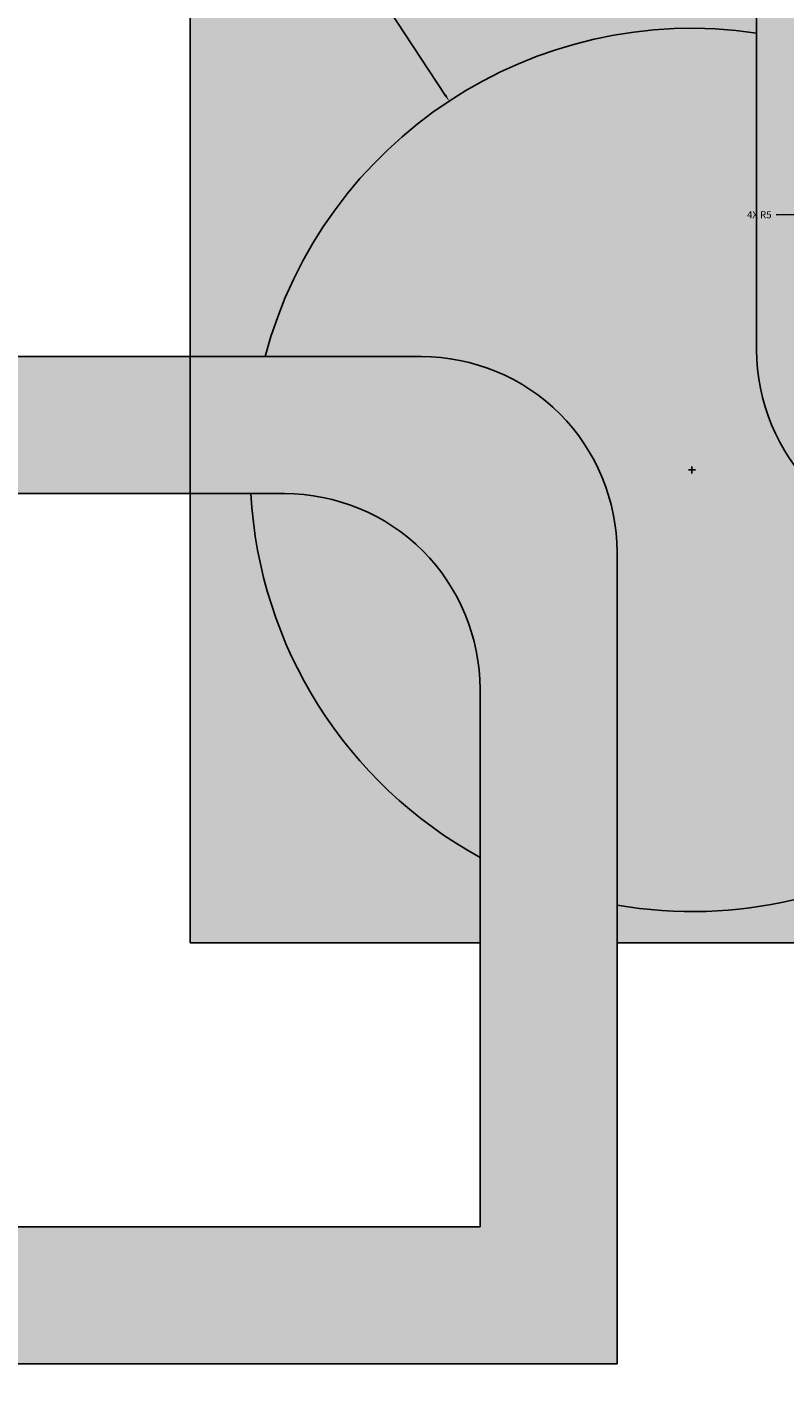
# Model space of a CAD drawing. Units: millimetres. Extents: x -11 to 280, y -4 to 208.
# Tile 30 of 55: x 170 to 189, y 54 to 88. Entities that reach past the tile are written whole.
import ezdxf

# ---------------------------------------------------------------- set-up
doc = ezdxf.new("R2010")
doc.units = ezdxf.units.MM
for name, color, linetype, lineweight in [('M-DIMS', 2, 'Continuous', 18), ('M-HYDR-PRES', 7, 'Continuous', 25), ('M-HYDR-RETN', 7, 'Continuous', 25), ('M-HYDR-VALV', 7, 'Continuous', 25), ('M-HYDR-VALV-PATT', 252, 'Continuous', 13)]:
    doc.layers.add(name, color=color, linetype=linetype, lineweight=lineweight)
doc.layers.add('M-HYDR-PRES-PATT', color=240, linetype='Continuous', lineweight=13, true_color=0xed1f24)
doc.layers.add('M-HYDR-RETN-PATT', color=114, linetype='Continuous', lineweight=13, true_color=0x139b48)
doc.styles.get("Standard").update_dxf_attribs({"font": 'arial.ttf'})
doc.dimstyles.get("Standard").update_dxf_attribs({"dimtxt": 0.18, "dimasz": 0.18, "dimexe": 0.18, "dimexo": 0.0625, "dimgap": 0.09, "dimtad": 0, "dimtih": 1, "dimtoh": 1, "dimdec": 4, "dimzin": 0, "dimdsep": 46, "dimtxsty": 'Standard', "dimcen": 0.09, "dimadec": 0, "dimazin": 0, "dimtfac": 1, "dimtdec": 4, "dimtofl": 0, "dimtmove": 0, "dimatfit": 3, "dimfxl": 1, "dimtolj": 1, "dimtzin": 0, "dimarcsym": 0})

# ---------------------------------------------------------------- blocks, each defined once
blk = doc.blocks.new('*D4')
at = {"layer": 'Defpoints', "color": 0, "transparency": 16777216}
for p in [(4.763, 84.426), (266.035, 51.733), (266.035, -3.415)]:
    blk.add_point(p, dxfattribs=at)
at = {"layer": 'M-DIMS', "color": 0, "lineweight": -2, "transparency": 16777216}
for p, q in [((4.763, 84.364), (4.763, -3.595)), ((266.035, 51.67), (266.035, -3.595)), ((4.943, -3.415), (134.934, -3.415)), ((265.855, -3.415), (135.864, -3.415))]:
    blk.add_line(p, q, dxfattribs=at)
at = {"layer": 'M-DIMS', "color": 0, "transparency": 16777216}
for points in [[(4.943, -3.385), (4.943, -3.445), (4.763, -3.415)], [(265.855, -3.385), (265.855, -3.445), (266.035, -3.415)]]:
    blk.add_solid(points, dxfattribs=at)
at = {"layer": 'M-DIMS', "color": 0, "transparency": 16777216, "insert": (135.399, -3.415), "char_height": 0.18, "attachment_point": 5}
blk.add_mtext('\\A1;261.27', dxfattribs=at)
blk = doc.blocks.new('*D5')
at = {"layer": 'Defpoints', "color": 0, "transparency": 16777216}
for p in [(24.759, 192.645), (-10.087, 11.435), (261.686, 11.435)]:
    blk.add_point(p, dxfattribs=at)
at = {"layer": 'M-DIMS', "color": 0, "lineweight": -2, "transparency": 16777216}
for p, q in [((24.696, 192.645), (-10.267, 192.645)), ((-10.087, 192.465), (-10.087, 102.222)), ((-10.087, 11.615), (-10.087, 101.858)), ((261.624, 11.435), (-10.267, 11.435))]:
    blk.add_line(p, q, dxfattribs=at)
at = {"layer": 'M-DIMS', "color": 0, "transparency": 16777216}
for points in [[(-10.117, 192.465), (-10.057, 192.465), (-10.087, 192.645)], [(-10.117, 11.615), (-10.057, 11.615), (-10.087, 11.435)]]:
    blk.add_solid(points, dxfattribs=at)
at = {"layer": 'M-DIMS', "color": 0, "transparency": 16777216, "insert": (-10.087, 102.04), "char_height": 0.18, "attachment_point": 5}
blk.add_mtext('\\A1;181.2', dxfattribs=at)
blk = doc.blocks.new('*D18')
at = {"layer": 'Defpoints', "color": 0, "transparency": 16777216}
for p in [(173.804, 207.495), (173.804, 65.064), (151.022, 43.599)]:
    blk.add_point(p, dxfattribs=at)
at = {"layer": 'M-DIMS', "color": 0, "lineweight": -2, "transparency": 16777216}
for p, q in [((151.022, 43.662), (151.022, 207.675)), ((151.202, 207.495), (162.017, 207.495)), ((173.624, 207.495), (162.808, 207.495)), ((173.804, 65.126), (173.804, 207.675))]:
    blk.add_line(p, q, dxfattribs=at)
at = {"layer": 'M-DIMS', "color": 0, "transparency": 16777216}
for points in [[(151.202, 207.525), (151.202, 207.465), (151.022, 207.495)], [(173.624, 207.525), (173.624, 207.465), (173.804, 207.495)]]:
    blk.add_solid(points, dxfattribs=at)
at = {"layer": 'M-DIMS', "color": 0, "transparency": 16777216, "insert": (162.413, 207.495), "char_height": 0.18, "attachment_point": 5}
blk.add_mtext('\\A1;22.78', dxfattribs=at)
blk = doc.blocks.new('*D20')
at = {"layer": 'Defpoints', "color": 0, "transparency": 16777216}
for p in [(231.68, 207.495), (151.022, 43.599), (231.68, 43.599)]:
    blk.add_point(p, dxfattribs=at)
at = {"layer": 'M-DIMS', "color": 0, "lineweight": -2, "transparency": 16777216}
for p, q in [((151.022, 43.662), (151.022, 207.675)), ((151.202, 207.495), (190.957, 207.495)), ((231.5, 207.495), (191.745, 207.495)), ((231.68, 43.662), (231.68, 207.675))]:
    blk.add_line(p, q, dxfattribs=at)
at = {"layer": 'M-DIMS', "color": 0, "transparency": 16777216}
for points in [[(151.202, 207.525), (151.202, 207.465), (151.022, 207.495)], [(231.5, 207.525), (231.5, 207.465), (231.68, 207.495)]]:
    blk.add_solid(points, dxfattribs=at)
at = {"layer": 'M-DIMS', "color": 0, "transparency": 16777216, "insert": (191.351, 207.495), "char_height": 0.18, "attachment_point": 5}
blk.add_mtext('\\A1;80.66', dxfattribs=at)
blk = doc.blocks.new('*D29')
at = {"layer": 'Defpoints', "color": 0, "transparency": 16777216}
for p in [(180.42, 86.567), (186.62, 77.144)]:
    blk.add_point(p, dxfattribs=at)
at = {"layer": 'M-DIMS', "color": 0, "lineweight": -2, "transparency": 16777216}
for p, q in [((176.52, 92.221), (176.7, 92.221)), ((176.7, 92.221), (180.321, 86.718)), ((186.53, 77.144), (186.71, 77.144)), ((186.62, 77.054), (186.62, 77.234))]:
    blk.add_line(p, q, dxfattribs=at)
at = {"layer": 'M-DIMS', "color": 0, "transparency": 16777216}
blk.add_solid([(180.346, 86.734), (180.296, 86.701), (180.42, 86.567)], dxfattribs=at)
at = {"layer": 'M-DIMS', "color": 0, "transparency": 16777216, "insert": (175.843, 92.221), "char_height": 0.18, "attachment_point": 5}
blk.add_mtext('\\A1;4X R11.28', dxfattribs=at)
blk = doc.blocks.new('*D31')
at = {"layer": 'Defpoints', "color": 0, "transparency": 16777216}
for p in [(191.775, 83.68), (196.774, 83.71)]:
    blk.add_point(p, dxfattribs=at)
at = {"layer": 'M-DIMS', "color": 0, "lineweight": -2, "transparency": 16777216}
for p, q in [((188.775, 83.662), (191.595, 83.679)), ((196.684, 83.71), (196.864, 83.71)), ((196.774, 83.62), (196.774, 83.8))]:
    blk.add_line(p, q, dxfattribs=at)
at = {"layer": 'M-DIMS', "color": 0, "transparency": 16777216}
blk.add_solid([(191.594, 83.709), (191.595, 83.649), (191.775, 83.68)], dxfattribs=at)
at = {"layer": 'M-DIMS', "color": 0, "transparency": 16777216, "insert": (188.342, 83.662), "char_height": 0.18, "attachment_point": 5}
blk.add_mtext('\\A1;4X R5', dxfattribs=at)

msp = doc.modelspace()

# ---------------------------------------------------------------- hatches: boundary and pattern name
at = {"layer": 'M-HYDR-PRES-PATT'}
h = msp.add_hatch(color=256, dxfattribs=at)
h.set_gradient(color1=(237, 31, 36), color2=(237, 31, 36), tint=1)
h.paths.add_polyline_path([(232.2, 133.1228), (228.7, 133.1228), (228.7, 108.8141), (102.7646, 108.8141), (102.7646, 105.3141), (232.2, 105.3141)])
h.paths.add_polyline_path([(128.8433, 105.3141), (125.3433, 105.3141), (125.3433, 91.7099, 1), (128.8433, 91.7099)])
h.paths.add_polyline_path([(229.1617, 78.7098), (196.7745, 78.7098, -0.4142136), (191.7745, 83.7098), (191.7745, 105.3141), (188.2745, 105.3141), (188.2745, 80.2098, 0.4142136), (193.2745, 75.2098), (225.6617, 75.2098), (225.6617, 43.5991), (229.1617, 43.5991)])
h.paths.add_polyline_path([(102.7646, 110.3704), (95.5776, 110.3704), (95.5776, 103.9022), (102.7646, 103.9022)])
h.paths.add_polyline_path([(100.7059, 107.2502), (99.1711, 106.3641), (99.1711, 106.8641), (97.1711, 106.8641), (97.1711, 107.6363), (99.1711, 107.6363), (99.1711, 108.1363)], flags=16)
h.paths.add_polyline_path([(234.6119, 138.4081), (226.5106, 138.4081), (226.5106, 133.1228), (234.6119, 133.1228)])
h.paths.add_polyline_path([(231.1963, 135.7055), (230.2965, 134.1786), (229.4241, 135.7213), (229.9241, 135.7168), (229.9418, 137.7167), (230.7141, 137.7099), (230.6963, 135.71)], flags=16)
at = {"layer": 'M-HYDR-RETN-PATT'}
h = msp.add_hatch(color=256, dxfattribs=at)
h.set_gradient(color1=(19, 155, 72), color2=(19, 155, 72), tint=1)
h.paths.add_polyline_path([(17.9701, 159.0814), (29.2015, 159.0814), (29.2015, 162.5814), (14.4701, 162.5814), (14.4701, 98.0213), (17.9701, 98.0213)])
h.paths.add_polyline_path([(17.9701, 84.4261), (14.4701, 84.4261), (14.4701, 54.3099), (156.2446, 54.3099), (156.2446, 57.8099), (17.9701, 57.8099)])
h.paths.add_polyline_path([(120.5137, 74.3991), (17.9701, 74.3991), (17.9701, 70.8991), (120.5137, 70.8991)], flags=17)
h.paths.add_polyline_path([(184.7092, 75.04, 0.4142136), (179.7092, 80.04), (156.2446, 80.04), (156.2446, 57.8099), (156.2446, 54.3099), (156.2446, 43.5991), (159.7446, 43.5991), (159.7446, 57.8099), (159.7446, 76.54), (176.2092, 76.54, -0.4142136), (181.2092, 71.54), (181.2092, 57.8099), (159.7446, 57.8099), (159.7446, 54.3099), (184.7092, 54.3099)])
at = {"layer": 'M-HYDR-VALV-PATT'}
h = msp.add_hatch(color=256, dxfattribs=at)
h.set_gradient(color1=(153, 27, 30), color2=(153, 27, 30), tint=1)
h.paths.add_polyline_path([(131.8437, 88.2421, -0.3394543), (132.5849, 89.208), (121.2548, 86.1721, -0.4931454), (122.5137, 85.2062, -0.3394543), (121.7725, 84.2403), (133.1025, 87.2762, -0.4931454)])
h.paths.add_polyline_path([(133.1025, 83.1351, -0.4931454), (131.8437, 84.101, -0.3394543), (132.5849, 85.0669), (121.2548, 82.031, -0.4931454), (122.5137, 81.0651, -0.3394543), (121.7725, 80.0992)])
h.paths.add_polyline_path([(133.1025, 78.994, -0.4931454), (131.8437, 79.9599, -0.3394543), (132.5849, 80.9258), (121.2548, 77.8899, -0.4931454), (122.5137, 76.924, -0.3394543), (121.7725, 75.9581)])
h.paths.add_polyline_path([(197.7905, 78.7098), (200.0003, 78.7098), (200.0003, 89.3873), (191.7745, 89.3873), (191.7745, 87.1776, -0.2439164)])
h.paths.add_polyline_path([(200.0003, 65.0638), (200.0003, 75.2098), (197.7325, 75.2098, -0.4135811), (184.7092, 66.0277), (184.7092, 65.0638)])
h.paths.add_polyline_path([(181.2092, 65.0638), (181.2092, 67.2471, -0.2598454), (175.3563, 76.54), (173.8038, 76.54), (173.8038, 65.0638)])
h.paths.add_polyline_path([(188.2745, 88.3022), (188.2745, 89.3873), (173.8038, 89.3873), (173.8038, 80.04), (175.7181, 80.04, -0.3816661)])
h = msp.add_hatch(color=256, dxfattribs=at)
h.set_gradient(color1=(205, 105, 40), color2=(34, 52, 110), tint=1, name='INVCYLINDER')
h.paths.add_polyline_path([(188.2745, 80.2098), (188.2745, 88.3022, 0.3816661), (175.7181, 80.04), (179.7092, 80.04, -0.4142136), (184.7092, 75.04), (184.7092, 66.0277, 0.4135811), (197.7325, 75.2098), (193.2745, 75.2098, -0.4142136)])
h.paths.add_polyline_path([(176.2092, 76.54), (175.3563, 76.54, 0.2598454), (181.2092, 67.2471), (181.2092, 71.54, 0.4142136)])
h.paths.add_polyline_path([(196.7745, 78.7098), (197.7905, 78.7098, 0.2439164), (191.7745, 87.1776), (191.7745, 83.7098, 0.4142136)])

# ---------------------------------------------------------------- linework, layer by layer
at = {"layer": 'M-HYDR-PRES'}
msp.add_lwpolyline([(188.2745, 105.3141), (188.2745, 80.2098, 0.4142136), (193.2745, 75.2098), (225.6617, 75.2098), (225.6617, 43.5991)], format="xyb", dxfattribs=at)
at = {"layer": 'M-HYDR-RETN'}
msp.add_lwpolyline([(159.7446, 54.3099), (184.7092, 54.3099), (184.7092, 75.04, 0.4142136), (179.7092, 80.04), (156.2446, 80.04), (156.2446, 57.8099)], format="xyb", dxfattribs=at)
msp.add_lwpolyline([(159.7446, 57.8099), (181.2092, 57.8099), (181.2092, 71.54, 0.4142136), (176.2092, 76.54), (159.7446, 76.54)], format="xyb", close=True, dxfattribs=at)
at = {"layer": 'M-HYDR-VALV'}
for points in [[(173.8038, 80.04), (173.8038, 89.3873), (188.2745, 89.3873)], [(181.2092, 65.0638), (173.8038, 65.0638), (173.8038, 76.54)], [(200.0003, 75.2098), (200.0003, 65.0638), (184.7092, 65.0638)]]:
    msp.add_lwpolyline(points, dxfattribs=at)
for start, end in [(81.565, 165.12565), (183.07195, 241.33562), (260.24776, 350.12401)]:
    msp.add_arc((186.6199, 77.1445), 11.2798, start, end, dxfattribs=at)

# ---------------------------------------------------------------- dimensions: what is measured, and where the dimension line sits
at = {"layer": 'M-DIMS'}
for base, p1, p2, picture, middle in [((173.8038, 207.495), (151.0217, 43.5991), (173.8038, 65.0638), '*D18', (162.4127, 207.495)), ((231.6803, 207.495), (151.0217, 43.5991), (231.6803, 43.5991), '*D20', (191.351, 207.495)), ((266.0352, -3.4154), (4.7635, 84.4261), (266.0352, 51.7328), '*D4', (135.3993, -3.4154))]:
    dim = msp.add_linear_dim(base=base, p1=p1, p2=p2, dimstyle='Standard', override={"dimdec": 2, "dimlfac": 1, "dimrnd": 0, "dimzin": 0, "dimdsep": 46, "dimlunit": 2}, dxfattribs=at)
    dim.commit()
    dim.dimension.update_dxf_attribs({"geometry": picture, "text_midpoint": middle})
dim = msp.add_linear_dim(base=(-10.0865, 11.4346), p1=(24.7588, 192.645), p2=(261.6863, 11.4346), angle=90, dimstyle='Standard', override={"dimdec": 1, "dimlfac": 1, "dimrnd": 0, "dimzin": 0, "dimdsep": 46, "dimlunit": 2}, dxfattribs=at)
dim.commit()
dim.dimension.update_dxf_attribs({"geometry": '*D5', "text_midpoint": (-10.0865, 102.0398)})
for center, mpoint, override, picture, middle in [((186.6199, 77.1445), (180.4197, 86.5674), {"dimdec": 2, "dimlfac": 1, "dimrnd": 0, "dimzin": 0, "dimdsep": 46, "dimlunit": 2}, '*D29', (175.8426, 92.2211)), ((196.7745, 83.7098), (191.7746, 83.6801), {"dimdec": 0, "dimlfac": 1, "dimrnd": 0, "dimzin": 0, "dimdsep": 46, "dimlunit": 2}, '*D31', (188.7746, 83.6623))]:
    dim = msp.add_radius_dim(center=center, mpoint=mpoint, text='4X <>', dimstyle='Standard', override=override, dxfattribs=at)
    dim.commit()
    dim.dimension.update_dxf_attribs({"geometry": picture, "text_midpoint": middle, "dimtype": 164})

doc.saveas('drawing.dxf')
